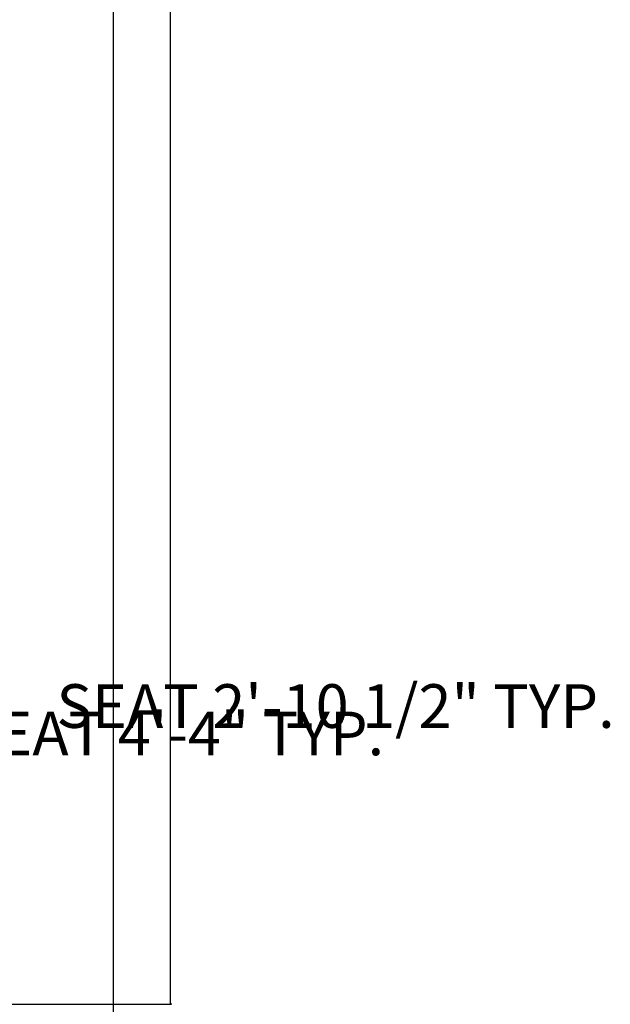
# Model space of a CAD drawing. Units: inches. Extents: x -11 to 443, y 65 to 743.
# Tile 6 of 10: x 335 to 443, y 212 to 392. Entities that reach past the tile are written whole.
import ezdxf

# ---------------------------------------------------------------- set-up
doc = ezdxf.new("R2010")
doc.units = ezdxf.units.IN
doc.header["$MEASUREMENT"] = 0
doc.layers.add('A-ANNO-DIMS', color=2, linetype='Continuous', lineweight=18)
doc.styles.get("Standard").update_dxf_attribs({"font": 'italic8.shx'})
doc.dimstyles.get("Standard").update_dxf_attribs({"dimtxt": 8, "dimasz": 0.18, "dimexe": 0.18, "dimexo": 0.0625, "dimgap": 0.09, "dimtad": 0, "dimtih": 1, "dimtoh": 1, "dimzin": 0, "dimdsep": 46, "dimlunit": 3, "dimtxsty": 'Standard', "dimblk": 'CLOSEDBLANK', "dimcen": 0.09, "dimclrd": 6, "dimclre": 5, "dimclrt": 4, "dimadec": 0, "dimazin": 0, "dimtfac": 1, "dimtofl": 0, "dimtmove": 0, "dimatfit": 3, "dimfxl": 1, "dimtolj": 1, "dimtzin": 0, "dimarcsym": 0})

# ---------------------------------------------------------------- blocks, each defined once
blk = doc.blocks.new('_ClosedBlank')
at = {"color": 0, "linetype": 'ByBlock', "lineweight": -2}
for p, q in [((-1, 0.167), (0, 0)), ((-1, 0.167), (-1, -0.167)), ((0, 0), (-1, -0.167))]:
    blk.add_line(p, q, dxfattribs=at)
blk = doc.blocks.new('*D6')
at = {"layer": 'A-ANNO-DIMS', "color": 0, "lineweight": -2, "transparency": 16777216}
for p, q in [((332.27, 706.92), (352.4, 706.92)), ((352.22, 706.74), (352.22, 411.77)), ((352.22, 107.1), (352.22, 402.07)), ((332.27, 106.92), (352.4, 106.92))]:
    blk.add_line(p, q, dxfattribs=at)
at = {"layer": 'Defpoints', "color": 0, "lineweight": 100, "transparency": 16777216}
for p in [(332.21, 706.92), (332.21, 106.92), (352.22, 106.92)]:
    blk.add_point(p, dxfattribs=at)
at = {"layer": 'A-ANNO-DIMS', "color": 0, "lineweight": -2, "transparency": 16777216, "xscale": 0.18, "yscale": 0.18, "zscale": 0.18}
for p, rotation in [((352.22, 706.92), 90), ((352.22, 106.92), 270)]:
    blk.add_blockref('_ClosedBlank', p, dxfattribs=dict(at, rotation=rotation))
at = {"layer": 'A-ANNO-DIMS', "color": 0, "transparency": 16777216, "insert": (352.22, 406.92), "char_height": 8, "attachment_point": 5}
blk.add_mtext("\\A1;50'", dxfattribs=at)
blk = doc.blocks.new('*D32')
at = {"layer": 'A-ANNO-DIMS', "color": 5, "lineweight": -2, "transparency": 16777216}
for p, q in [((223.42, 253.79), (223.42, 261.7)), ((275.39, 253.79), (275.39, 261.7))]:
    blk.add_line(p, q, dxfattribs=at)
at = {"layer": 'A-ANNO-DIMS', "color": 6, "lineweight": -2, "transparency": 16777216}
for p, q in [((223.6, 261.52), (275.21, 261.52)), ((275.39, 261.52), (275.57, 261.52))]:
    blk.add_line(p, q, dxfattribs=at)
at = {"layer": 'Defpoints', "color": 0, "lineweight": 100, "transparency": 16777216}
for p in [(275.39, 261.52), (223.42, 253.72), (275.39, 253.72)]:
    blk.add_point(p, dxfattribs=at)
at = {"layer": 'A-ANNO-DIMS', "color": 6, "lineweight": -2, "transparency": 16777216, "xscale": 0.18, "yscale": 0.18, "zscale": 0.18, "rotation": 180}
blk.add_blockref('_ClosedBlank', (223.42, 261.52), dxfattribs=at)
at = {"layer": 'A-ANNO-DIMS', "color": 6, "lineweight": -2, "transparency": 16777216, "xscale": 0.18, "yscale": 0.18, "zscale": 0.18}
blk.add_blockref('_ClosedBlank', (275.39, 261.52), dxfattribs=at)
at = {"layer": 'A-ANNO-DIMS', "color": 4, "transparency": 16777216, "insert": (349.75, 261.52), "char_height": 8, "attachment_point": 5}
blk.add_mtext('\\A1;LOVESEAT 4\'-4" TYP.', dxfattribs=at)
blk = doc.blocks.new('*D34')
at = {"layer": 'A-ANNO-DIMS', "color": 5, "lineweight": -2, "transparency": 16777216}
for p, q in [((283.03, 261.45), (283.03, 266.72)), ((317.39, 261.45), (317.39, 266.72))]:
    blk.add_line(p, q, dxfattribs=at)
at = {"layer": 'A-ANNO-DIMS', "color": 6, "lineweight": -2, "transparency": 16777216}
for p, q in [((283.21, 266.54), (317.21, 266.54)), ((317.39, 266.54), (317.57, 266.54))]:
    blk.add_line(p, q, dxfattribs=at)
at = {"layer": 'Defpoints', "color": 0, "lineweight": 100, "transparency": 16777216}
for p in [(317.39, 266.54), (283.03, 261.39), (317.39, 261.39)]:
    blk.add_point(p, dxfattribs=at)
at = {"layer": 'A-ANNO-DIMS', "color": 6, "lineweight": -2, "transparency": 16777216, "xscale": 0.18, "yscale": 0.18, "zscale": 0.18, "rotation": 180}
blk.add_blockref('_ClosedBlank', (283.03, 266.54), dxfattribs=at)
at = {"layer": 'A-ANNO-DIMS', "color": 6, "lineweight": -2, "transparency": 16777216, "xscale": 0.18, "yscale": 0.18, "zscale": 0.18}
blk.add_blockref('_ClosedBlank', (317.39, 266.54), dxfattribs=at)
at = {"layer": 'A-ANNO-DIMS', "color": 4, "transparency": 16777216, "insert": (392.9, 266.54), "char_height": 8, "attachment_point": 5}
blk.add_mtext('\\A1;SEAT 2\'-10 1/2" TYP.', dxfattribs=at)
blk = doc.blocks.new('*D36')
at = {"layer": 'A-ANNO-DIMS', "color": 5, "lineweight": -2, "transparency": 16777216}
for p, q in [((323.27, 625.92), (362.85, 625.92)), ((323.27, 211.92), (362.85, 211.92))]:
    blk.add_line(p, q, dxfattribs=at)
at = {"layer": 'A-ANNO-DIMS', "color": 6, "lineweight": -2, "transparency": 16777216}
for p, q in [((362.67, 625.74), (362.67, 423.77)), ((362.67, 212.1), (362.67, 414.07))]:
    blk.add_line(p, q, dxfattribs=at)
at = {"layer": 'Defpoints', "color": 0, "lineweight": 100, "transparency": 16777216}
for p in [(323.21, 625.92), (362.67, 625.92), (323.21, 211.92)]:
    blk.add_point(p, dxfattribs=at)
at = {"layer": 'A-ANNO-DIMS', "color": 6, "lineweight": -2, "transparency": 16777216, "xscale": 0.18, "yscale": 0.18, "zscale": 0.18}
for p, rotation in [((362.67, 625.92), 90), ((362.67, 211.92), 270)]:
    blk.add_blockref('_ClosedBlank', p, dxfattribs=dict(at, rotation=rotation))
at = {"layer": 'A-ANNO-DIMS', "color": 4, "transparency": 16777216, "insert": (362.67, 418.92), "char_height": 8, "attachment_point": 5}
blk.add_mtext('\\A1;34\'-6"', dxfattribs=at)

msp = doc.modelspace()

# ---------------------------------------------------------------- dimensions: what is measured, and where the dimension line sits
at = {"layer": 'A-ANNO-DIMS'}
for base, p1, p2, override, picture, middle in [((352.221, 106.92), (332.209, 706.92), (332.209, 106.92), {"dimclrd": 0, "dimclre": 0, "dimclrt": 0}, '*D6', (352.221, 406.92)), ((362.669, 625.92), (323.209, 211.92), (323.209, 625.92), {"dimdec": 1, "dimlfac": 1, "dimrnd": 0, "dimzin": 1, "dimdsep": 46, "dimlunit": 4, "dimfrac": 2}, '*D36', (362.669, 418.92))]:
    dim = msp.add_linear_dim(base=base, p1=p1, p2=p2, angle=90, dimstyle='Standard', override=override, dxfattribs=at)
    dim.commit()
    dim.dimension.update_dxf_attribs({"geometry": picture, "text_midpoint": middle})
for base, p1, p2, text, picture, middle in [((317.389, 266.543), (283.033, 261.39), (317.389, 261.39), 'SEAT <> TYP.', '*D34', (392.897, 266.543)), ((275.388, 261.518), (223.42, 253.723), (275.388, 253.723), 'LOVESEAT <> TYP.', '*D32', (349.753, 261.518))]:
    dim = msp.add_linear_dim(base=base, p1=p1, p2=p2, text=text, dimstyle='Standard', override={"dimdec": 1, "dimlfac": 1, "dimrnd": 0, "dimzin": 1, "dimdsep": 46, "dimlunit": 4, "dimfrac": 2}, dxfattribs=at)
    dim.commit()
    dim.dimension.update_dxf_attribs({"geometry": picture, "text_midpoint": middle})

doc.saveas('drawing.dxf')
